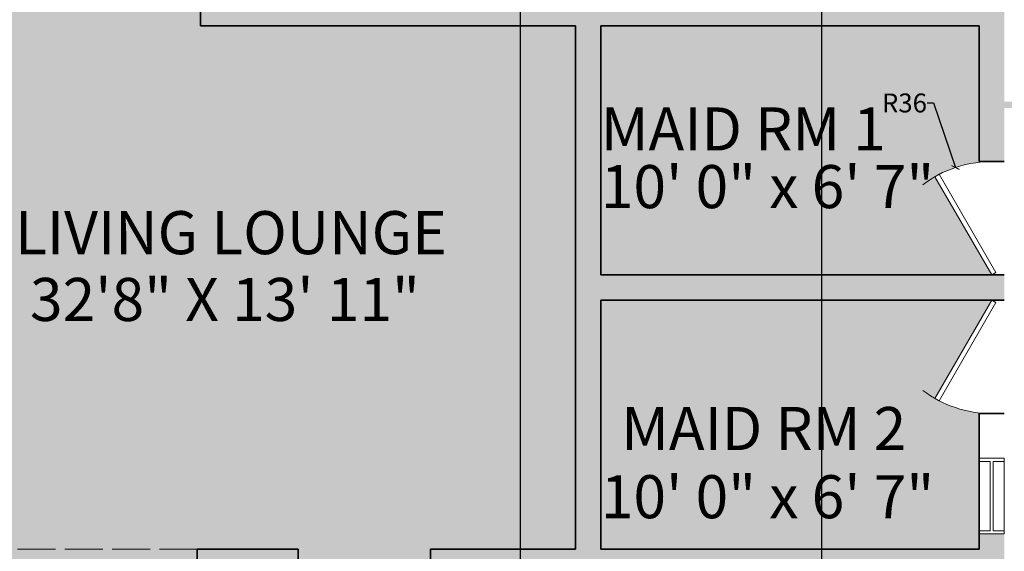
# Model space of a CAD drawing. Units: inches. Extents: x 1704 to 6393, y -157 to 1172.
# Tile 86 of 122: x 2293 to 2605, y 372 to 540. Entities that reach past the tile are written whole.
import ezdxf

# ---------------------------------------------------------------- set-up
doc = ezdxf.new("R2010")
doc.units = ezdxf.units.IN
doc.header["$MEASUREMENT"] = 0
doc.linetypes.add('ACAD_ISO02W100', pattern=[15, 12, -3])
for name, color, linetype, lineweight in [('A-ANNO-DIMS', 7, 'Continuous', 13), ('A-AREA-IDEN', 7, 'Continuous', 18), ('A-WALL-OVHD', 8, 'ACAD_ISO02W100', 13), ('A-WALL-PATT', 7, 'Continuous', 13), ('DOORS', 160, 'Continuous', 18), ('WALLS', 7, 'Continuous', 35), ('WINDOWS', 2, 'Continuous', 18)]:
    doc.layers.add(name, color=color, linetype=linetype, lineweight=lineweight)
doc.layers.add('A-FLOR-PATT', color=7, linetype='Continuous', lineweight=13, true_color=0xf2f2f2)
doc.styles.get("Standard").update_dxf_attribs({"font": 'arial.ttf'})
doc.dimstyles.get("Standard").update_dxf_attribs({"dimtxt": 6, "dimasz": 2, "dimexe": 0.18, "dimexo": 0.0625, "dimgap": 0.09, "dimtad": 0, "dimtih": 1, "dimtoh": 1, "dimdec": 1, "dimzin": 0, "dimdsep": 46, "dimlunit": 3, "dimtxsty": 'Standard', "dimblk": 'ARCHTICK', "dimcen": 0.09, "dimadec": 0, "dimazin": 0, "dimtfac": 1, "dimtdec": 1, "dimtofl": 0, "dimtmove": 0, "dimatfit": 3, "dimfxl": 1, "dimtolj": 1, "dimtzin": 0, "dimarcsym": 0})

# ---------------------------------------------------------------- blocks, each defined once
blk = doc.blocks.new('Door - Left Hung 36 in.')
blk.add_lwpolyline([(0.75, -1.3), (0, 0), (31.18, 18), (31.93, 16.7)], close=True)
blk.add_arc((0, 0), 36, 0, 37.3101)
blk = doc.blocks.new('WIN-VENT-24')
for p, q in [((0, 0), (0, 24)), ((0, 24), (8, 24)), ((0, 23), (3.5, 23)), ((3.5, 23), (3.5, 1)), ((4.5, 23), (8, 23)), ((4.5, 23), (4.5, 1)), ((8, 24), (8, 0)), ((3.5, 1), (0, 1)), ((8, 1), (4.5, 1)), ((8, 0), (0, 0))]:
    blk.add_line(p, q)
blk = doc.blocks.new('_ArchTick')
at = {"color": 0, "linetype": 'ByBlock', "const_width": 0.15}
blk.add_lwpolyline([(-0.5, -0.5), (0.5, 0.5)], dxfattribs=at)
blk = doc.blocks.new('*D58')
at = {"layer": 'A-ANNO-DIMS', "color": 0, "lineweight": -2, "transparency": 16777216}
for p, q in [((2200.54, 354.32), (2200.54, 357)), ((2200.54, 356.82), (2217.62, 356.82)), ((2217.62, 354.32), (2217.62, 357)), ((2217.62, 356.82), (2219.62, 356.82))]:
    blk.add_line(p, q, dxfattribs=at)
at = {"layer": 'Defpoints', "color": 0, "lineweight": -3, "transparency": 16777216}
for p in [(2217.62, 356.82), (2200.54, 354.26), (2217.62, 354.26)]:
    blk.add_point(p, dxfattribs=at)
at = {"layer": 'A-ANNO-DIMS', "color": 0, "lineweight": -2, "transparency": 16777216, "xscale": 2, "yscale": 2, "zscale": 2, "rotation": 180}
blk.add_blockref('_ArchTick', (2200.54, 356.82), dxfattribs=at)
at = {"layer": 'A-ANNO-DIMS', "color": 0, "lineweight": -2, "transparency": 16777216, "xscale": 2, "yscale": 2, "zscale": 2}
blk.add_blockref('_ArchTick', (2217.62, 356.82), dxfattribs=at)
at = {"layer": 'A-ANNO-DIMS', "color": 0, "transparency": 16777216, "insert": (2262.58, 356.82), "char_height": 6, "attachment_point": 5}
blk.add_mtext('\\A1;PALLA CHAIR 17 TYP.', dxfattribs=at)
blk = doc.blocks.new('*D93')
at = {"layer": 'A-ANNO-DIMS', "color": 0, "lineweight": -2, "transparency": 16777216}
for p, q in [((2605.29, 895.21), (1829.7, 895.21)), ((1829.88, 895.21), (1829.88, 495.87)), ((1829.88, 90.21), (1829.88, 489.56)), ((2605.29, 90.21), (1829.7, 90.21))]:
    blk.add_line(p, q, dxfattribs=at)
at = {"layer": 'Defpoints', "color": 0, "lineweight": -3, "transparency": 16777216}
for p in [(2605.35, 895.21), (1829.88, 90.21), (2605.35, 90.21)]:
    blk.add_point(p, dxfattribs=at)
at = {"layer": 'A-ANNO-DIMS', "color": 0, "lineweight": -2, "transparency": 16777216, "xscale": 2, "yscale": 2, "zscale": 2}
for p, rotation in [((1829.88, 895.21), 90), ((1829.88, 90.21), 270)]:
    blk.add_blockref('_ArchTick', p, dxfattribs=dict(at, rotation=rotation))
at = {"layer": 'A-ANNO-DIMS', "color": 0, "transparency": 16777216, "insert": (1829.88, 492.71), "char_height": 6, "attachment_point": 5}
blk.add_mtext('\\A1;805', dxfattribs=at)
blk = doc.blocks.new('*D105')
at = {"layer": 'A-ANNO-DIMS', "color": 0, "lineweight": -2, "transparency": 16777216}
for p, q in [((2451.74, 615.15), (2451.74, -64.97)), ((2547.35, 615.15), (2547.35, -64.97)), ((2451.74, -64.79), (2489.91, -64.79)), ((2547.35, -64.79), (2509.18, -64.79))]:
    blk.add_line(p, q, dxfattribs=at)
at = {"layer": 'Defpoints', "color": 0, "lineweight": -3, "transparency": 16777216}
for p in [(2451.74, 615.21), (2547.35, 615.21), (2547.35, -64.79)]:
    blk.add_point(p, dxfattribs=at)
at = {"layer": 'A-ANNO-DIMS', "color": 0, "lineweight": -2, "transparency": 16777216, "xscale": 2, "yscale": 2, "zscale": 2, "rotation": 180}
blk.add_blockref('_ArchTick', (2451.74, -64.79), dxfattribs=at)
at = {"layer": 'A-ANNO-DIMS', "color": 0, "lineweight": -2, "transparency": 16777216, "xscale": 2, "yscale": 2, "zscale": 2}
blk.add_blockref('_ArchTick', (2547.35, -64.79), dxfattribs=at)
at = {"layer": 'A-ANNO-DIMS', "color": 0, "transparency": 16777216, "insert": (2499.54, -64.79), "char_height": 6, "attachment_point": 5}
blk.add_mtext('\\A1;95.61', dxfattribs=at)
blk = doc.blocks.new('*D137')
at = {"layer": 'A-ANNO-DIMS', "color": 0, "lineweight": -2, "transparency": 16777216}
for p, q in [((2580.92, 513.79), (2582.92, 513.79)), ((2582.92, 513.79), (2589.83, 493.32)), ((2601.26, 459.21), (2601.44, 459.21)), ((2601.35, 459.12), (2601.35, 459.3))]:
    blk.add_line(p, q, dxfattribs=at)
at = {"layer": 'Defpoints', "color": 0, "lineweight": -3, "transparency": 16777216}
for p in [(2589.83, 493.32), (2601.35, 459.21)]:
    blk.add_point(p, dxfattribs=at)
at = {"layer": 'A-ANNO-DIMS', "color": 0, "lineweight": -2, "transparency": 16777216, "xscale": 2, "yscale": 2, "zscale": 2, "rotation": 288.6552347934461}
blk.add_blockref('_ArchTick', (2589.83, 493.32), dxfattribs=at)
at = {"layer": 'A-ANNO-DIMS', "color": 0, "transparency": 16777216, "insert": (2573.67, 513.79), "char_height": 6, "attachment_point": 5}
blk.add_mtext('\\A1;R36', dxfattribs=at)

msp = doc.modelspace()

# ---------------------------------------------------------------- hatches: boundary and pattern name
at = {"layer": 'A-FLOR-PATT', "transparency": 33554528}
h = msp.add_hatch(color=256, dxfattribs=at)
h.dxf.hatch_style = 1
h.paths.add_polyline_path([(2325.349, 863.213), (2325.349, 887.213), (2263.349, 887.213), (2167.349, 887.213), (2081.349, 887.213), (2081.349, 719.213), (2277.349, 719.213), (2277.349, 711.213), (2277.349, 372.213), (2349.349, 372.213), (2381.349, 372.213), (2381.349, 364.213), (2353.349, 364.213), (2353.349, 270.213), (2381.349, 270.213), (2381.349, 266.213), (2357.349, 266.213), (2357.349, 98.213), (2381.349, 98.213), (2385.181, 98.213), (2386.482, 98.213), (2424.215, 98.213), (2425.516, 98.213), (2429.349, 98.213), (2597.349, 98.213), (2597.349, 146.213), (2597.349, 218.213), (2597.349, 266.213), (2423.349, 266.213), (2423.349, 270.213), (2473.349, 270.213), (2473.349, 294.213), (2477.349, 294.213), (2477.349, 270.213), (2547.349, 270.213), (2547.349, 364.213), (2477.349, 364.213), (2477.349, 318.213), (2473.349, 318.213), (2473.349, 364.213), (2423.349, 364.213), (2423.349, 372.213), (2469.349, 372.213), (2469.349, 459.213), (2469.349, 538.213), (2350.349, 538.213), (2350.349, 565.713), (2358.349, 565.713), (2358.349, 545.213), (2420.349, 545.213), (2420.349, 610.213), (2358.349, 610.213), (2358.349, 589.713), (2350.349, 589.713), (2350.349, 615.213), (2425.349, 615.213), (2425.349, 607.213), (2425.349, 546.213), (2469.349, 546.213), (2514.349, 546.213), (2514.349, 607.213), (2449.349, 607.213), (2449.349, 615.213), (2451.738, 615.213), (2451.738, 659.213), (2427.738, 659.213), (2427.738, 665.213), (2367.738, 665.213), (2367.738, 667.213), (2367.738, 711.213), (2325.349, 711.213), (2325.349, 719.213), (2325.349, 755.213), (2325.349, 763.213)])
h.paths.add_polyline_path([(2233.858, 822.533, -0.187247), (2233.858, 809.14), (2231.697, 808.804, 0.0848928), (2233.131, 814.486), (2230.424, 814.486, -0.1042581), (2228.553, 808.313), (2217.751, 807.156, -0.2222222), (2217.751, 824.517), (2228.553, 823.359, -0.1042581), (2230.424, 817.186), (2233.131, 817.186, 0.0848928), (2231.697, 822.868)], flags=16)
h.paths.add_polyline_path([(2213.621, 833.197), (2213.621, 798.475), (2156.048, 798.475), (2156.048, 833.197)], flags=16)
h.paths.add_polyline_path([(2203.932, 848.099), (2205.089, 837.296, -0.2222222), (2187.728, 837.296), (2188.885, 848.099, -0.1042581), (2195.058, 849.969), (2195.058, 852.676, 0.0848928), (2189.377, 851.242), (2189.712, 853.404, -0.187247), (2203.105, 853.404), (2203.44, 851.242, 0.0848928), (2197.759, 852.676), (2197.759, 849.969, -0.1042581)], flags=16)
h.paths.add_polyline_path([(2181.941, 837.296, -0.2222222), (2164.58, 837.296), (2165.737, 848.099, -0.1042581), (2171.91, 849.969), (2171.91, 852.676, 0.0848928), (2166.229, 851.242), (2166.564, 853.404, -0.187247), (2179.957, 853.404), (2180.292, 851.242, 0.0848928), (2174.611, 852.676), (2174.611, 849.969, -0.1042581), (2180.784, 848.099)], flags=16)
h.paths.add_polyline_path([(2205.089, 794.376), (2203.932, 783.574, -0.1042581), (2197.759, 781.703), (2197.759, 778.996, 0.0848928), (2203.44, 780.43), (2203.105, 778.269, -0.187247), (2189.712, 778.269), (2189.377, 780.43, 0.0848928), (2195.058, 778.996), (2195.058, 781.703, -0.1042581), (2188.885, 783.574), (2187.728, 794.376, -0.2222222)], flags=16)
h.paths.add_polyline_path([(2181.941, 794.376), (2180.784, 783.574, -0.1042581), (2174.611, 781.703), (2174.611, 778.996, 0.0848928), (2180.292, 780.43), (2179.957, 778.269, -0.187247), (2166.564, 778.269), (2166.229, 780.43, 0.0848928), (2171.91, 778.996), (2171.91, 781.703, -0.1042581), (2165.737, 783.574), (2164.58, 794.376, -0.2222222)], flags=16)
h.paths.add_polyline_path([(2151.918, 807.156), (2141.116, 808.313, -0.1042581), (2139.245, 814.486), (2136.539, 814.486, 0.0848928), (2137.972, 808.804), (2135.811, 809.14, -0.187247), (2135.811, 822.533), (2137.972, 822.868, 0.0848928), (2136.539, 817.186), (2139.245, 817.186, -0.1042581), (2141.116, 823.359), (2151.918, 824.517, -0.2222222)], flags=16)
h.paths.add_polyline_path([(2357.868, 363.41), (2358.814, 363.41, 0.7537605)], flags=16)
h.paths.add_polyline_path([(2372.241, 363.117), (2372.248, 363.117), (2372.248, 363.343), (2371.302, 363.343), (2371.302, 363.139, -1.3603913)], flags=16)
h.paths.add_polyline_path([(2371.309, 272.716), (2371.302, 272.716), (2371.302, 272.49), (2372.248, 272.49), (2372.248, 272.693, -1.3603913)], flags=16)
h.paths.add_polyline_path([(2357.875, 272.716), (2357.868, 272.716), (2357.868, 272.49), (2358.814, 272.49), (2358.814, 272.693, -1.3603913)], flags=16)
h.paths.add_polyline_path([(2353.769, 363.074), (2376.347, 363.074), (2376.347, 272.759), (2353.769, 272.759)], flags=16)
h.paths.add_polyline_path([(2354.772, 362.07), (2375.344, 362.07), (2375.344, 273.762), (2354.772, 273.762)], flags=0)
h.paths.add_polyline_path([(2357.868, 363.343), (2358.814, 363.343), (2358.814, 363.117), (2357.868, 363.117)], flags=16)
h.paths.add_polyline_path([(2359.288, 359.184), (2359.288, 360.063), (2370.828, 360.063), (2370.828, 359.184), (2374.332, 359.184), (2374.332, 358.464), (2372.835, 358.464), (2372.835, 357.541), (2374.332, 357.541), (2374.332, 356.82), (2372.835, 356.82), (2372.835, 355.898), (2374.332, 355.898), (2374.332, 355.177), (2372.835, 355.177), (2372.835, 354.254), (2374.332, 354.254), (2374.332, 353.534), (2372.835, 353.534), (2372.835, 352.611), (2374.332, 352.611), (2374.332, 351.89), (2372.835, 351.89), (2372.835, 350.968), (2374.332, 350.968), (2374.332, 350.247), (2372.835, 350.247), (2372.835, 349.324), (2374.332, 349.324), (2374.332, 348.604), (2372.835, 348.604), (2372.835, 347.681), (2374.332, 347.681), (2374.332, 346.96), (2372.835, 346.96), (2372.835, 346.038), (2374.332, 346.038), (2374.332, 345.317), (2372.835, 345.317), (2372.835, 344.395), (2374.332, 344.395), (2374.332, 343.674), (2372.835, 343.674), (2372.835, 342.751), (2374.332, 342.751), (2374.332, 342.03), (2372.835, 342.03), (2372.835, 341.108), (2374.332, 341.108), (2374.332, 340.387), (2372.835, 340.387), (2372.835, 339.465), (2374.332, 339.465), (2374.332, 338.744), (2372.835, 338.744), (2372.835, 337.821), (2374.332, 337.821), (2374.332, 337.1), (2372.835, 337.1), (2372.835, 336.178), (2374.332, 336.178), (2374.332, 335.457), (2372.835, 335.457), (2372.835, 334.535), (2374.332, 334.535), (2374.332, 333.814), (2372.835, 333.814), (2372.835, 332.891), (2374.332, 332.891), (2374.332, 332.171), (2372.835, 332.171), (2372.835, 331.248), (2374.332, 331.248), (2374.332, 330.527), (2372.835, 330.527), (2372.835, 329.605), (2374.332, 329.605), (2374.332, 328.884), (2372.835, 328.884), (2372.835, 327.961), (2374.332, 327.961), (2374.332, 327.241), (2372.835, 327.241), (2372.835, 326.318), (2374.332, 326.318), (2374.332, 325.597), (2372.835, 325.597), (2372.835, 324.675), (2374.332, 324.675), (2374.332, 323.954), (2372.835, 323.954), (2372.835, 323.031), (2374.332, 323.031), (2374.332, 322.311), (2372.835, 322.311), (2372.835, 321.388), (2374.332, 321.388), (2374.332, 320.667), (2372.835, 320.667), (2372.835, 319.745), (2374.332, 319.745), (2374.332, 319.024), (2372.835, 319.024), (2372.835, 318.102), (2374.332, 318.102), (2374.332, 317.381), (2372.835, 317.381), (2372.835, 316.458), (2374.332, 316.458), (2374.332, 315.737), (2372.835, 315.737), (2372.835, 314.815), (2374.332, 314.815), (2374.332, 314.094), (2372.835, 314.094), (2372.835, 313.172), (2374.332, 313.172), (2374.332, 312.451), (2372.835, 312.451), (2372.835, 311.528), (2374.332, 311.528), (2374.332, 310.807), (2372.835, 310.807), (2372.835, 309.885), (2374.332, 309.885), (2374.332, 309.164), (2372.835, 309.164), (2372.835, 308.242), (2374.332, 308.242), (2374.332, 307.521), (2372.835, 307.521), (2372.835, 306.598), (2374.332, 306.598), (2374.332, 305.878), (2372.835, 305.878), (2372.835, 304.955), (2374.332, 304.955), (2374.332, 304.234), (2372.835, 304.234), (2372.835, 303.312), (2374.332, 303.312), (2374.332, 302.591), (2372.835, 302.591), (2372.835, 301.668), (2374.332, 301.668), (2374.332, 300.948), (2372.835, 300.948), (2372.835, 300.025), (2374.332, 300.025), (2374.332, 299.304), (2372.835, 299.304), (2372.835, 298.382), (2374.332, 298.382), (2374.332, 297.661), (2372.835, 297.661), (2372.835, 296.738), (2374.332, 296.738), (2374.332, 296.018), (2372.835, 296.018), (2372.835, 295.095), (2374.332, 295.095), (2374.332, 294.374), (2372.835, 294.374), (2372.835, 293.452), (2374.332, 293.452), (2374.332, 292.731), (2372.835, 292.731), (2372.835, 291.809), (2374.332, 291.809), (2374.332, 291.088), (2372.835, 291.088), (2372.835, 290.165), (2374.332, 290.165), (2374.332, 289.444), (2372.835, 289.444), (2372.835, 288.522), (2374.332, 288.522), (2374.332, 287.801), (2372.835, 287.801), (2372.835, 286.879), (2374.332, 286.879), (2374.332, 286.158), (2372.835, 286.158), (2372.835, 285.235), (2374.332, 285.235), (2374.332, 284.514), (2372.835, 284.514), (2372.835, 283.592), (2374.332, 283.592), (2374.332, 282.871), (2372.835, 282.871), (2372.835, 281.949), (2374.332, 281.949), (2374.332, 281.228), (2372.835, 281.228), (2372.835, 280.305), (2374.332, 280.305), (2374.332, 279.585), (2372.835, 279.585), (2372.835, 278.662), (2374.332, 278.662), (2374.332, 277.941), (2372.835, 277.941), (2372.835, 277.019), (2374.332, 277.019), (2374.332, 276.298), (2370.828, 276.298), (2370.828, 275.769), (2359.288, 275.769), (2359.288, 276.298), (2355.784, 276.298), (2355.784, 277.019), (2357.281, 277.019), (2357.281, 277.941), (2355.784, 277.941), (2355.784, 278.662), (2357.281, 278.662), (2357.281, 279.585), (2355.784, 279.585), (2355.784, 280.305), (2357.281, 280.305), (2357.281, 281.228), (2355.784, 281.228), (2355.784, 281.949), (2357.281, 281.949), (2357.281, 282.871), (2355.784, 282.871), (2355.784, 283.592), (2357.281, 283.592), (2357.281, 284.514), (2355.784, 284.514), (2355.784, 285.235), (2357.281, 285.235), (2357.281, 286.158), (2355.784, 286.158), (2355.784, 286.879), (2357.281, 286.879), (2357.281, 287.801), (2355.784, 287.801), (2355.784, 288.522), (2357.281, 288.522), (2357.281, 289.444), (2355.784, 289.444), (2355.784, 290.165), (2357.281, 290.165), (2357.281, 291.088), (2355.784, 291.088), (2355.784, 291.809), (2357.281, 291.809), (2357.281, 292.731), (2355.784, 292.731), (2355.784, 293.452), (2357.281, 293.452), (2357.281, 294.374), (2355.784, 294.374), (2355.784, 295.095), (2357.281, 295.095), (2357.281, 296.018), (2355.784, 296.018), (2355.784, 296.738), (2357.281, 296.738), (2357.281, 297.661), (2355.784, 297.661), (2355.784, 298.382), (2357.281, 298.382), (2357.281, 299.304), (2355.784, 299.304), (2355.784, 300.025), (2357.281, 300.025), (2357.281, 300.948), (2355.784, 300.948), (2355.784, 301.668), (2357.281, 301.668), (2357.281, 302.591), (2355.784, 302.591), (2355.784, 303.312), (2357.281, 303.312), (2357.281, 304.234), (2355.784, 304.234), (2355.784, 304.955), (2357.281, 304.955), (2357.281, 305.878), (2355.784, 305.878), (2355.784, 306.598), (2357.281, 306.598), (2357.281, 307.521), (2355.784, 307.521), (2355.784, 308.242), (2357.281, 308.242), (2357.281, 309.164), (2355.784, 309.164), (2355.784, 309.885), (2357.281, 309.885), (2357.281, 310.807), (2355.784, 310.807), (2355.784, 311.528), (2357.281, 311.528), (2357.281, 312.451), (2355.784, 312.451), (2355.784, 313.172), (2357.281, 313.172), (2357.281, 314.094), (2355.784, 314.094), (2355.784, 314.815), (2357.281, 314.815), (2357.281, 315.737), (2355.784, 315.737), (2355.784, 316.458), (2357.281, 316.458), (2357.281, 317.381), (2355.784, 317.381), (2355.784, 318.102), (2357.281, 318.102), (2357.281, 319.024), (2355.784, 319.024), (2355.784, 319.745), (2357.281, 319.745), (2357.281, 320.667), (2355.784, 320.667), (2355.784, 321.388), (2357.281, 321.388), (2357.281, 322.311), (2355.784, 322.311), (2355.784, 323.031), (2357.281, 323.031), (2357.281, 323.954), (2355.784, 323.954), (2355.784, 324.675), (2357.281, 324.675), (2357.281, 325.597), (2355.784, 325.597), (2355.784, 326.318), (2357.281, 326.318), (2357.281, 327.241), (2355.784, 327.241), (2355.784, 327.961), (2357.281, 327.961), (2357.281, 328.884), (2355.784, 328.884), (2355.784, 329.605), (2357.281, 329.605), (2357.281, 330.527), (2355.784, 330.527), (2355.784, 331.248), (2357.281, 331.248), (2357.281, 332.171), (2355.784, 332.171), (2355.784, 332.891), (2357.281, 332.891), (2357.281, 333.814), (2355.784, 333.814), (2355.784, 334.535), (2357.281, 334.535), (2357.281, 335.457), (2355.784, 335.457), (2355.784, 336.178), (2357.281, 336.178), (2357.281, 337.1), (2355.784, 337.1), (2355.784, 337.821), (2357.281, 337.821), (2357.281, 338.744), (2355.784, 338.744), (2355.784, 339.465), (2357.281, 339.465), (2357.281, 340.387), (2355.784, 340.387), (2355.784, 341.108), (2357.281, 341.108), (2357.281, 342.03), (2355.784, 342.03), (2355.784, 342.751), (2357.281, 342.751), (2357.281, 343.674), (2355.784, 343.674), (2355.784, 344.395), (2357.281, 344.395), (2357.281, 345.317), (2355.784, 345.317), (2355.784, 346.038), (2357.281, 346.038), (2357.281, 346.96), (2355.784, 346.96), (2355.784, 347.681), (2357.281, 347.681), (2357.281, 348.604), (2355.784, 348.604), (2355.784, 349.324), (2357.281, 349.324), (2357.281, 350.247), (2355.784, 350.247), (2355.784, 350.968), (2357.281, 350.968), (2357.281, 351.89), (2355.784, 351.89), (2355.784, 352.611), (2357.281, 352.611), (2357.281, 353.534), (2355.784, 353.534), (2355.784, 354.254), (2357.281, 354.254), (2357.281, 355.177), (2355.784, 355.177), (2355.784, 355.898), (2357.281, 355.898), (2357.281, 356.82), (2355.784, 356.82), (2355.784, 357.541), (2357.281, 357.541), (2357.281, 358.464), (2355.784, 358.464), (2355.784, 359.184)], flags=0)
h = msp.add_hatch(color=256, dxfattribs=at)
h.dxf.hatch_style = 1
h.paths.add_polyline_path([(2601.349, 451.213), (2597.349, 451.213), (2477.349, 451.213), (2477.349, 372.213), (2597.349, 372.213), (2597.349, 415.436, -0.0929107), (2584.663, 419.313), (2584.648, 419.286), (2583.349, 420.036)])
h.paths.add_polyline_path([(2583.349, 490.39), (2584.648, 491.14), (2584.663, 491.113, -0.0929107), (2597.349, 494.99), (2597.349, 538.213), (2477.349, 538.213), (2477.349, 459.213), (2597.349, 459.213), (2601.349, 459.213)])
h.paths.add_polyline_path([(2587.444, 580.63), (2587.431, 580.607), (2586.349, 581.232), (2601.349, 607.213), (2532.349, 607.213), (2518.349, 607.213), (2518.349, 542.213), (2597.349, 542.213), (2597.349, 577.481, -0.0872676)])
h.paths.add_polyline_path([(2597.349, 711.213), (2551.349, 711.213), (2551.349, 615.213), (2597.349, 615.213), (2601.349, 615.213), (2586.349, 641.194), (2587.431, 641.819), (2587.444, 641.796, -0.1210664), (2601.349, 645.213), (2597.349, 645.213)])
h.paths.add_polyline_path([(2547.349, 659.213), (2532.738, 659.213), (2532.738, 615.213), (2547.349, 615.213)])
h.paths.add_polyline_path([(2547.349, 711.213), (2532.738, 711.213), (2532.738, 667.213), (2547.349, 667.213)])
h.paths.add_polyline_path([(2357.349, 755.213), (2325.349, 755.213), (2325.349, 719.213), (2357.349, 719.213)])
h.paths.add_polyline_path([(2451.738, 711.213), (2428.738, 711.213), (2428.738, 667.213), (2451.738, 667.213)])
h.paths.add_polyline_path([(2427.738, 711.213), (2418.738, 711.213), (2418.738, 667.213), (2427.738, 667.213)])
h.paths.add_polyline_path([(2417.738, 711.213), (2408.738, 711.213), (2408.738, 667.213), (2417.738, 667.213)])
h.paths.add_polyline_path([(2407.738, 711.213), (2398.738, 711.213), (2398.738, 667.213), (2407.738, 667.213)])
h.paths.add_polyline_path([(2397.738, 711.213), (2388.738, 711.213), (2388.738, 667.213), (2397.738, 667.213)])
h.paths.add_polyline_path([(2387.738, 711.213), (2378.738, 711.213), (2378.738, 667.213), (2387.738, 667.213)])
h.paths.add_polyline_path([(2377.738, 711.213), (2368.738, 711.213), (2368.738, 667.213), (2377.738, 667.213)])
h.paths.add_polyline_path([(2461.738, 711.213), (2452.738, 711.213), (2452.738, 667.213), (2461.738, 667.213)])
h.paths.add_polyline_path([(2471.738, 711.213), (2462.738, 711.213), (2462.738, 667.213), (2471.738, 667.213)])
h.paths.add_polyline_path([(2481.738, 711.213), (2472.738, 711.213), (2472.738, 667.213), (2481.738, 667.213)])
h.paths.add_polyline_path([(2491.738, 711.213), (2482.738, 711.213), (2482.738, 667.213), (2491.738, 667.213)])
h.paths.add_polyline_path([(2501.738, 711.213), (2492.738, 711.213), (2492.738, 667.213), (2501.738, 667.213)])
h.paths.add_polyline_path([(2511.738, 711.213), (2502.738, 711.213), (2502.738, 667.213), (2511.738, 667.213)])
h.paths.add_polyline_path([(2521.738, 711.213), (2512.738, 711.213), (2512.738, 667.213), (2521.738, 667.213)])
h.paths.add_polyline_path([(2531.738, 711.213), (2522.738, 711.213), (2522.738, 667.213), (2531.738, 667.213)])
h.paths.add_polyline_path([(2522.738, 711.213), (2521.738, 711.213), (2521.738, 667.213), (2522.738, 667.213)])
h.paths.add_polyline_path([(2512.738, 711.213), (2511.738, 711.213), (2511.738, 667.213), (2512.738, 667.213)])
h.paths.add_polyline_path([(2531.738, 659.213), (2522.738, 659.213), (2522.738, 615.213), (2531.738, 615.213)])
h.paths.add_polyline_path([(2521.738, 659.213), (2512.738, 659.213), (2512.738, 615.213), (2521.738, 615.213)])
h.paths.add_polyline_path([(2511.738, 659.213), (2502.738, 659.213), (2502.738, 615.213), (2511.738, 615.213)])
h.paths.add_polyline_path([(2501.738, 659.213), (2492.738, 659.213), (2492.738, 615.213), (2501.738, 615.213)])
h.paths.add_polyline_path([(2491.738, 659.213), (2482.738, 659.213), (2482.738, 615.213), (2491.738, 615.213)])
h.paths.add_polyline_path([(2481.738, 659.213), (2472.738, 659.213), (2472.738, 615.213), (2481.738, 615.213)])
h.paths.add_polyline_path([(2471.738, 659.213), (2462.738, 659.213), (2462.738, 615.213), (2471.738, 615.213)])
h.paths.add_polyline_path([(2461.738, 659.213), (2452.738, 659.213), (2452.738, 615.213), (2461.738, 615.213)])
h.paths.add_polyline_path([(2545.349, 665.213), (2451.738, 665.213), (2451.738, 661.213), (2545.349, 661.213)], flags=17)
h.paths.add_polyline_path([(2547.349, 667.213), (2532.738, 667.213), (2451.738, 667.213), (2451.738, 665.213), (2545.349, 665.213), (2545.349, 661.213), (2451.738, 661.213), (2451.738, 659.213), (2547.349, 659.213)])
h = msp.add_hatch(color=256, dxfattribs=at)
h.dxf.hatch_style = 1
h.paths.add_polyline_path([(2349.349, 372.213), (2277.349, 372.213), (2277.349, 364.213), (2349.349, 364.213)])
h.paths.add_polyline_path([(2277.349, 372.213), (2273.349, 372.213), (2273.349, 364.213), (2277.349, 364.213)])
h.paths.add_polyline_path([(2277.349, 364.213), (2273.349, 364.213), (2273.349, 202.213), (2277.349, 202.213)])
h.paths.add_polyline_path([(2277.349, 538.213), (2273.349, 538.213), (2273.349, 372.213), (2277.349, 372.213)])
h.paths.add_polyline_path([(2277.349, 629.213), (2273.349, 629.213), (2273.349, 545.213), (2277.349, 545.213)])
h.paths.add_polyline_path([(2277.349, 711.213), (2273.349, 711.213), (2273.349, 631.213), (2277.349, 631.213)])
h.paths.add_polyline_path([(2277.349, 631.213), (2273.349, 631.213), (2273.349, 629.213), (2277.349, 629.213)])
at = {"layer": 'A-WALL-PATT', "transparency": 33554643}
h = msp.add_hatch(color=256, dxfattribs=at)
h.dxf.hatch_style = 1
h.paths.add_polyline_path([(2167.349, 895.213), (2073.349, 895.213), (2073.349, 887.213), (2081.349, 887.213), (2167.349, 887.213)])
h.paths.add_polyline_path([(2465.349, 895.213), (2273.349, 895.213), (2273.349, 903.213), (2263.349, 903.213), (2263.349, 895.213), (2263.349, 887.213), (2325.349, 887.213), (2325.349, 863.213), (2333.349, 863.213), (2333.349, 887.213), (2465.349, 887.213)])
h.paths.add_polyline_path([(2533.349, 895.213), (2513.349, 895.213), (2513.349, 887.213), (2513.349, 861.213), (2517.349, 861.213), (2517.349, 887.213), (2533.349, 887.213)])
h.paths.add_polyline_path([(2605.349, 895.213), (2581.349, 895.213), (2581.349, 887.213), (2597.349, 887.213), (2597.349, 854.213), (2605.349, 854.213)])
h.paths.add_polyline_path([(2605.349, 752.213), (2629.349, 752.213), (2629.349, 716.213), (2605.349, 716.213), (2605.349, 712.213), (2719.349, 712.213), (2719.349, 716.213), (2631.349, 716.213), (2631.349, 754.213), (2605.349, 754.213), (2605.349, 794.213), (2597.349, 794.213), (2597.349, 787.213), (2517.349, 787.213), (2517.349, 813.213), (2513.349, 813.213), (2513.349, 783.213), (2517.349, 783.213), (2597.349, 783.213), (2597.349, 719.213), (2517.349, 719.213), (2517.349, 753.213), (2513.349, 753.213), (2513.349, 719.213), (2365.349, 719.213), (2365.349, 763.213), (2325.349, 763.213), (2325.349, 755.213), (2357.349, 755.213), (2357.349, 719.213), (2325.349, 719.213), (2325.349, 711.213), (2547.349, 711.213), (2547.349, 615.213), (2449.349, 615.213), (2449.349, 607.213), (2514.349, 607.213), (2514.349, 546.213), (2439.349, 546.213), (2425.349, 546.213), (2425.349, 607.213), (2425.349, 615.213), (2350.349, 615.213), (2350.349, 589.713), (2358.349, 589.713), (2358.349, 610.213), (2420.349, 610.213), (2420.349, 545.213), (2358.349, 545.213), (2358.349, 565.713), (2350.349, 565.713), (2350.349, 538.213), (2469.349, 538.213), (2469.349, 459.213), (2469.349, 372.213), (2423.349, 372.213), (2423.349, 364.213), (2473.349, 364.213), (2473.349, 318.213), (2477.349, 318.213), (2477.349, 364.213), (2547.349, 364.213), (2547.349, 352.213), (2549.349, 352.213), (2549.349, 364.213), (2597.349, 364.213), (2597.349, 328.213), (2549.349, 328.213), (2547.349, 328.213), (2547.349, 326.213), (2549.349, 326.213), (2597.349, 326.213), (2605.349, 326.213), (2605.349, 377.057), (2597.349, 377.057), (2597.349, 372.213), (2477.349, 372.213), (2477.349, 451.213), (2597.349, 451.213), (2605.349, 451.213), (2605.349, 459.213), (2597.349, 459.213), (2477.349, 459.213), (2477.349, 538.213), (2597.349, 538.213), (2597.349, 495.213), (2605.349, 495.213), (2605.349, 512.213), (2631.349, 512.213), (2631.349, 568.213), (2605.349, 568.213), (2605.349, 577.213), (2597.349, 577.213), (2597.349, 542.213), (2518.349, 542.213), (2518.349, 607.213), (2532.349, 607.213), (2605.349, 607.213), (2605.349, 615.213), (2597.349, 615.213), (2551.349, 615.213), (2551.349, 711.213), (2597.349, 711.213), (2597.349, 645.213), (2605.349, 645.213), (2605.349, 712.213), (2605.349, 716.213)])
h.paths.add_polyline_path([(2605.349, 566.213), (2629.349, 566.213), (2629.349, 514.213), (2605.349, 514.213)], flags=16)
h.paths.add_polyline_path([(2381.349, 372.213), (2349.349, 372.213), (2349.349, 202.213), (2337.349, 202.213), (2337.349, 194.213), (2349.349, 194.213), (2349.349, 90.213), (2349.349, 72.213), (2357.349, 72.213), (2357.349, 90.213), (2381.349, 90.213), (2381.349, 98.213), (2357.349, 98.213), (2357.349, 266.213), (2381.349, 266.213), (2381.349, 270.213), (2353.349, 270.213), (2353.349, 364.213), (2381.349, 364.213)])
h.paths.add_polyline_path([(2605.349, 302.213), (2597.349, 302.213), (2597.349, 270.213), (2477.349, 270.213), (2477.349, 294.213), (2473.349, 294.213), (2473.349, 270.213), (2423.349, 270.213), (2423.349, 266.213), (2597.349, 266.213), (2597.349, 218.213), (2605.349, 218.213)])
h.paths.add_polyline_path([(2605.349, 146.213), (2597.349, 146.213), (2597.349, 98.213), (2429.349, 98.213), (2429.349, 90.213), (2597.349, 90.213), (2597.349, 72.213), (2605.349, 72.213), (2605.349, 90.213)])
h.paths.add_polyline_path([(2225.349, 202.213), (2049.349, 202.213), (2049.349, 194.213), (2225.349, 194.213)])
h.paths.add_polyline_path([(2289.349, 202.213), (2277.349, 202.213), (2273.349, 202.213), (2269.516, 202.213), (2269.516, 194.213), (2273.349, 194.213), (2277.349, 194.213), (2289.349, 194.213)])
h.paths.add_polyline_path([(2273.349, 372.213), (2029.19, 372.213), (2029.19, 364.213), (2273.349, 364.213)])
h.paths.add_polyline_path([(2277.349, 545.213), (2213.349, 545.213), (2213.349, 573.213), (2205.349, 573.213), (2177.349, 573.213), (2177.349, 545.213), (2073.349, 545.213), (2073.349, 538.213), (2081.349, 538.213), (2277.349, 538.213)])
h.paths.add_polyline_path([(2181.349, 545.213), (2181.349, 569.213), (2205.349, 569.213), (2205.349, 545.213)], flags=16)
h.paths.add_polyline_path([(2277.349, 719.213), (2081.349, 719.213), (2073.349, 719.213), (2073.349, 711.213), (2154.575, 711.213), (2205.349, 711.213), (2205.349, 687.213), (2205.349, 629.213), (2213.349, 629.213), (2273.349, 629.213), (2273.349, 631.213), (2207.349, 631.213), (2207.349, 707.213), (2231.349, 707.213), (2231.349, 709.213), (2207.349, 709.213), (2207.349, 711.213), (2277.349, 711.213)])

# ---------------------------------------------------------------- linework, layer by layer
at = {"layer": 'A-WALL-OVHD'}
msp.add_line((2277.349, 372.213), (2349.349, 372.213), dxfattribs=at)
at = {"layer": 'WALLS'}
for p, q in [((2350.349, 538.213), (2350.349, 565.713)), ((2469.349, 538.213), (2350.349, 538.213)), ((2469.349, 459.213), (2469.349, 538.213)), ((2597.349, 538.213), (2477.349, 538.213)), ((2477.349, 459.213), (2477.349, 538.213)), ((2597.349, 495.213), (2597.349, 538.213)), ((2597.349, 495.213), (2605.349, 495.213)), ((2469.349, 372.213), (2469.349, 459.213)), ((2597.349, 459.213), (2477.349, 459.213)), ((2597.349, 459.213), (2605.349, 459.213)), ((2597.349, 451.213), (2477.349, 451.213)), ((2477.349, 372.213), (2477.349, 451.213)), ((2597.349, 451.213), (2605.349, 451.213)), ((2597.349, 372.213), (2597.349, 415.213)), ((2597.349, 415.213), (2605.349, 415.213)), ((2349.349, 202.213), (2349.349, 372.213)), ((2381.349, 372.213), (2349.349, 372.213)), ((2381.349, 364.213), (2381.349, 372.213)), ((2469.349, 372.213), (2423.349, 372.213)), ((2423.349, 364.213), (2423.349, 372.213)), ((2597.349, 372.213), (2477.349, 372.213))]:
    msp.add_line(p, q, dxfattribs=at)

# ---------------------------------------------------------------- block references
at = {"layer": 'DOORS', "rotation": 90.00000000000003}
msp.add_blockref('Door - Left Hung 36 in.', (2601.349, 459.213), dxfattribs=at)
at = {"layer": 'DOORS', "xscale": -1, "rotation": 90}
msp.add_blockref('Door - Left Hung 36 in.', (2601.349, 451.213), dxfattribs=at)
at = {"layer": 'WINDOWS'}
msp.add_blockref('WIN-VENT-24', (2597.349, 377.057), dxfattribs=at)

# ---------------------------------------------------------------- texts
at = {"layer": 'A-ANNO-DIMS'}
for s, p in [('10\' 0" x 6\' 7"', (2477.349, 480.414)), ('32\'8" X 13\' 11"', (2296.257, 444.609)), ('10\' 0" x 6\' 7"', (2477.349, 382.009))]:
    msp.add_text(s, height=13.6672, dxfattribs=at).set_placement(p)
at = {"layer": 'A-AREA-IDEN'}
for s, p in [('MAID RM 1', (2477.349, 498.713)), ('LIVING LOUNGE', (2291.5, 465.801)), ('MAID RM 2', (2483.789, 403.644))]:
    msp.add_text(s, height=13.6672, dxfattribs=at).set_placement(p)

# ---------------------------------------------------------------- dimensions: what is measured, and where the dimension line sits
at = {"layer": 'A-ANNO-DIMS'}
dim = msp.add_linear_dim(base=(1829.878, 90.213), p1=(2605.349, 895.213), p2=(2605.349, 90.213), angle=90, dimstyle='Standard', override={"dimdec": 0, "dimlfac": 1, "dimrnd": 0, "dimzin": 0, "dimdsep": 46, "dimlunit": 2}, dxfattribs=at)
dim.commit()
dim.dimension.update_dxf_attribs({"geometry": '*D93', "text_midpoint": (1829.878, 492.713)})
dim = msp.add_linear_dim(base=(2547.349, -64.787), p1=(2451.738, 615.213), p2=(2547.349, 615.213), dimstyle='Standard', override={"dimdec": 2, "dimlfac": 1, "dimrnd": 0, "dimzin": 0, "dimdsep": 46, "dimlunit": 2}, dxfattribs=at)
dim.commit()
dim.dimension.update_dxf_attribs({"geometry": '*D105', "text_midpoint": (2499.543, -64.787)})
dim = msp.add_radius_dim(center=(2601.349, 459.213), mpoint=(2589.833, 493.322), dimstyle='Standard', override={"dimdec": 0, "dimlfac": 1, "dimrnd": 0, "dimzin": 0, "dimdsep": 46, "dimlunit": 2}, dxfattribs=at)
dim.commit()
dim.dimension.update_dxf_attribs({"geometry": '*D137', "text_midpoint": (2573.667, 513.787), "dimtype": 164})
dim = msp.add_linear_dim(base=(2217.621, 356.821), p1=(2200.535, 354.258), p2=(2217.621, 354.258), text='PALLA CHAIR <> TYP.', dimstyle='Standard', override={"dimdec": 0, "dimlfac": 1, "dimrnd": 0, "dimzin": 0, "dimdsep": 46, "dimlunit": 2}, dxfattribs=at)
dim.commit()
dim.dimension.update_dxf_attribs({"geometry": '*D58', "text_midpoint": (2262.58, 356.821)})

doc.saveas('drawing.dxf')
